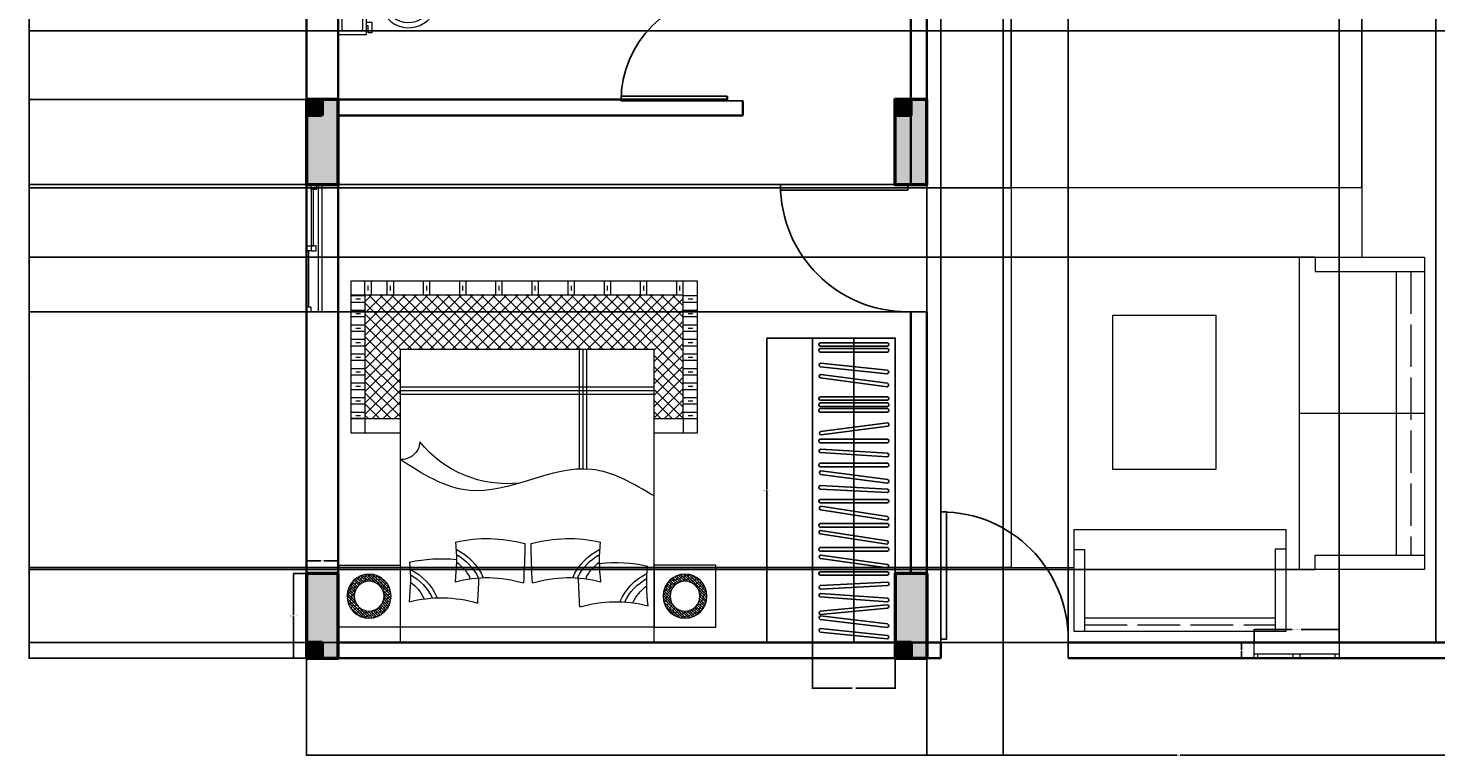
# Model space of a CAD drawing. Units: inches. Extents: x 393 to 993, y 153 to 660.
# Tile 1 of 6: x 393 to 791, y 153 to 359. Entities that reach past the tile are written whole.
import ezdxf

# ---------------------------------------------------------------- set-up
doc = ezdxf.new("R2010")
doc.units = ezdxf.units.IN
doc.header["$MEASUREMENT"] = 0
doc.linetypes.add('ACAD_ISO02W100', pattern=[15, 12, -3])
for name, color, linetype, lineweight in [('A-ANNO-DIMS', 2, 'Continuous', 18), ('A-COLS', 40, 'Continuous', 50), ('A-FLOR-CASE', 72, 'Continuous', 25), ('A-FLOR-FIXT', 9, 'Continuous', 18), ('A-FURN-HIDN', 72, 'ACAD_ISO02W100', 13), ('A-GLAZ', 4, 'Continuous', 20), ('A-WALL', 40, 'Continuous', 35), ('DOORS', 32, 'Continuous', 25), ('FURNITURE', 72, 'Continuous', 18)]:
    doc.layers.add(name, color=color, linetype=linetype, lineweight=lineweight)
doc.styles.get("Standard").update_dxf_attribs({"font": 'arial.ttf'})
doc.dimstyles.get("Standard").update_dxf_attribs({"dimtxt": 0.18, "dimasz": 0.18, "dimexe": 0.18, "dimexo": 0.0625, "dimgap": 0.09, "dimtad": 0, "dimtih": 1, "dimtoh": 1, "dimdec": 1, "dimzin": 0, "dimdsep": 46, "dimlunit": 3, "dimtxsty": 'Standard', "dimcen": 0.09, "dimadec": 0, "dimazin": 0, "dimtfac": 1, "dimtdec": 1, "dimtofl": 0, "dimtmove": 0, "dimatfit": 3, "dimfxl": 1, "dimtolj": 1, "dimtzin": 0, "dimarcsym": 0})

# ---------------------------------------------------------------- blocks, each defined once
blk = doc.blocks.new('W')
for p, q in [((518.15, 606.48), (554.15, 606.48)), ((518.15, 605.48), (554.15, 605.48))]:
    blk.add_line(p, q)
for points in [[(518.15, 609.91), (554.15, 609.91), (554.15, 600.91), (518.15, 600.91)], [(519.42, 609.91), (518.15, 609.91), (518.15, 608.51), (519.42, 608.51)], [(519.42, 609.91), (535.35, 609.91), (535.35, 609.3), (519.42, 609.3)], [(535.35, 609.91), (536.78, 609.91), (536.78, 608.51), (535.35, 608.51)], [(536.78, 608.51), (535.35, 608.51), (535.35, 607.12), (536.78, 607.12)], [(552.72, 608.51), (536.78, 608.51), (536.78, 607.91), (552.72, 607.91)], [(552.72, 608.51), (554.15, 608.51), (554.15, 607.12), (552.72, 607.12)]]:
    blk.add_lwpolyline(points, close=True)
blk = doc.blocks.new('*U3')
for p, q in [((0, 0), (0, -6)), ((40, 0), (40, -6))]:
    blk.add_line(p, q)
blk.add_lwpolyline([(0, 0), (0, 40), (1.75, 40), (1.75, 0)], close=True)
blk.add_arc((0, 0), 40, 0, 90)
blk = doc.blocks.new('GG')
for p, q in [((752.1, 182.21), (764.1, 182.21)), ((752.96, 182.21), (752.96, 180.91)), ((763, 180.91), (763, 182.21))]:
    blk.add_line(p, q)
for points in [[(740.1, 180.91), (740.1, 185.41), (764.1, 185.41), (764.1, 180.91), (740.1, 180.91), (740.1, 182.21), (752.1, 182.21)], [(740.1, 180.91), (741.16, 180.91), (741.16, 182.21)], [(752.1, 180.91), (751.16, 180.91), (751.16, 182.21)]]:
    blk.add_lwpolyline(points)
blk = doc.blocks.new('BED')
h = blk.add_hatch()
h.set_pattern_fill('ANSI38', color=256, scale=4.4)
h.paths.add_polyline_path([(503.33, 587.82, 1), (515.77, 587.82, 1)])
h.paths.add_polyline_path([(513.77, 587.82, -1), (505.33, 587.82, -1)], flags=16)
h = blk.add_hatch()
h.set_pattern_fill('ANSI38', color=256, scale=4.4)
h.paths.add_polyline_path([(592.69, 587.82, 1), (605.13, 587.82, 1)])
h.paths.add_polyline_path([(603.13, 587.82, -1), (594.69, 587.82, -1)], flags=16)
h = blk.add_hatch()
h.set_pattern_fill('ANSI37', color=256, scale=18)
h.paths.add_polyline_path([(518.29, 518.09), (518.29, 537.6), (508.38, 537.6), (508.38, 502.74), (598.4, 502.74), (598.4, 537.6), (590.17, 537.6), (590.17, 518.09)])
for p, q in [((569.1, 551.87), (569.1, 518.09)), ((570.1, 551.87), (570.1, 518.09)), ((571.1, 551.87), (571.1, 518.09)), ((508.38, 537.6), (508.38, 541.6)), ((598.4, 537.6), (598.4, 541.6)), ((508.38, 537.6), (504.38, 537.6)), ((504.38, 537.6), (508.38, 537.6)), ((598.4, 537.6), (602.4, 537.6)), ((504.38, 535.78), (508.38, 535.78)), ((505.75, 536.69), (507.09, 536.69)), ((598.4, 535.78), (602.4, 535.78)), ((599.77, 536.69), (601.11, 536.69)), ((504.38, 533.48), (508.38, 533.48)), ((504.38, 531.66), (508.38, 531.66)), ((505.75, 532.57), (507.09, 532.57)), ((518.29, 530.67), (590.17, 530.67)), ((518.29, 529.67), (590.17, 529.67)), ((598.4, 533.48), (602.4, 533.48)), ((598.4, 531.66), (602.4, 531.66)), ((599.77, 532.57), (601.11, 532.57)), ((504.38, 529.37), (508.38, 529.37)), ((504.38, 527.54), (508.38, 527.54)), ((505.75, 528.46), (507.09, 528.46)), ((518.29, 528.67), (590.17, 528.67)), ((598.4, 529.37), (602.4, 529.37)), ((598.4, 527.54), (602.4, 527.54)), ((599.77, 528.46), (601.11, 528.46)), ((504.38, 525.25), (508.38, 525.25)), ((504.38, 523.43), (508.38, 523.43)), ((505.75, 524.34), (507.09, 524.34)), ((598.4, 525.25), (602.4, 525.25)), ((598.4, 523.43), (602.4, 523.43)), ((599.77, 524.34), (601.11, 524.34)), ((504.38, 521.13), (508.38, 521.13)), ((504.38, 519.31), (508.38, 519.31)), ((505.75, 520.22), (507.09, 520.22)), ((598.4, 521.13), (602.4, 521.13)), ((598.4, 519.31), (602.4, 519.31)), ((599.77, 520.22), (601.11, 520.22)), ((504.38, 517.02), (508.38, 517.02)), ((504.38, 515.19), (508.38, 515.19)), ((505.75, 516.11), (507.09, 516.11)), ((598.4, 517.02), (602.4, 517.02)), ((598.4, 515.19), (602.4, 515.19)), ((599.77, 516.11), (601.11, 516.11)), ((504.38, 512.9), (508.38, 512.9)), ((504.38, 511.08), (508.38, 511.08)), ((505.75, 511.99), (507.09, 511.99)), ((598.4, 512.9), (602.4, 512.9)), ((598.4, 511.08), (602.4, 511.08)), ((599.77, 511.99), (601.11, 511.99)), ((504.38, 508.78), (508.38, 508.78)), ((504.38, 506.96), (508.38, 506.96)), ((505.75, 507.87), (507.09, 507.87)), ((598.4, 508.78), (602.4, 508.78)), ((598.4, 506.96), (602.4, 506.96)), ((599.77, 507.87), (601.11, 507.87)), ((504.38, 504.67), (508.38, 504.67)), ((504.38, 502.84), (508.38, 502.84)), ((508.38, 502.74), (504.38, 502.74)), ((505.75, 503.76), (507.09, 503.76)), ((508.38, 502.74), (508.38, 498.74)), ((510.2, 502.74), (510.2, 498.74)), ((514.7, 502.74), (514.7, 498.74)), ((516.52, 502.74), (516.52, 498.74)), ((524.93, 502.74), (524.93, 498.74)), ((526.76, 502.74), (526.76, 498.74)), ((535.17, 502.74), (535.17, 498.74)), ((536.99, 502.74), (536.99, 498.74)), ((545.4, 502.74), (545.4, 498.74)), ((547.22, 502.74), (547.22, 498.74)), ((555.64, 502.74), (555.64, 498.74)), ((557.46, 502.74), (557.46, 498.74)), ((565.87, 502.74), (565.87, 498.74)), ((567.69, 502.74), (567.69, 498.74)), ((576.11, 502.74), (576.11, 498.74)), ((577.93, 502.74), (577.93, 498.74)), ((586.34, 502.74), (586.34, 498.74)), ((588.16, 502.74), (588.16, 498.74)), ((596.58, 502.74), (596.58, 498.74)), ((598.4, 504.67), (602.4, 504.67)), ((598.4, 502.84), (602.4, 502.84)), ((598.4, 502.74), (598.4, 498.74)), ((599.77, 503.76), (601.11, 503.76)), ((509.29, 501.37), (509.29, 500.03)), ((515.61, 501.37), (515.61, 500.03)), ((525.84, 501.37), (525.84, 500.03)), ((536.08, 501.37), (536.08, 500.03)), ((546.31, 501.37), (546.31, 500.03)), ((556.55, 501.37), (556.55, 500.03)), ((566.78, 501.37), (566.78, 500.03)), ((577.02, 501.37), (577.02, 500.03)), ((587.25, 501.37), (587.25, 500.03)), ((597.49, 501.37), (597.49, 500.03))]:
    blk.add_line(p, q)
for points in [[(518.29, 600.91), (590.17, 600.91), (590.17, 518.09), (518.29, 518.09)], [(518.29, 600.91), (590.17, 600.91), (590.17, 596.58), (518.29, 596.58)], [(518.29, 596.58), (500.81, 596.58), (500.81, 579.05), (518.29, 579.05)], [(590.17, 596.58), (607.65, 596.58), (607.65, 579.05), (590.17, 579.05)]]:
    blk.add_lwpolyline(points, close=True)
for points in [[(590.17, 541.6), (602.4, 541.6), (602.4, 498.74), (504.38, 498.74), (504.38, 541.6), (518.29, 541.6)], [(590.17, 537.6), (598.4, 537.6), (598.4, 502.74), (508.38, 502.74), (508.38, 537.6), (518.29, 537.6)]]:
    blk.add_lwpolyline(points)
for centre, radius in [((509.55, 587.82), 6.22), ((598.91, 587.82), 6.22), ((509.55, 587.82), 4.22), ((598.91, 587.82), 4.22)]:
    blk.add_circle(centre, radius)
for centre, radius, start, end in [((529.91, 624.74), 36.45, 255.5916, 286.3549), ((470.26, 583.22), 50.97, 354.3497, 7.0055), ((355.3, 577.59), 185.28, 1.5729, 3.7686), ((754.03, 578.68), 185.28, 176.2314, 178.7587), ((579.42, 625.84), 36.45, 253.6451, 284.4084), ((595.11, 595.65), 15.87, 203.1669, 244.1569), ((595.11, 595.65), 14.59, 205.0537, 241.3945), ((595.75, 595.21), 12.82, 205.4838, 233.4213), ((639.07, 584.32), 50.97, 172.9945, 185.6503), ((514.22, 594.55), 15.87, 295.8431, 336.8331), ((514.22, 594.55), 14.59, 298.6055, 334.9463), ((513.58, 594.12), 12.82, 306.5787, 334.5162), ((542.93, 619.04), 36.45, 255.5916, 286.3549), ((483.27, 577.52), 50.97, 354.3497, 7.0055), ((527.24, 588.86), 15.87, 295.8431, 336.8331), ((527.24, 588.86), 14.59, 298.6055, 334.9463), ((526.6, 588.42), 12.82, 306.5787, 334.5162), ((368.32, 571.89), 185.28, 0.3263, 3.7686), ((740.67, 571.89), 185.28, 176.2314, 179.6737), ((566.06, 619.04), 36.45, 253.6451, 284.4084), ((581.75, 588.86), 15.87, 203.1669, 244.1569), ((581.75, 588.86), 14.59, 205.0537, 241.3945), ((582.39, 588.42), 12.82, 205.4838, 233.4213), ((625.71, 577.52), 50.97, 172.9945, 185.6503), ((529.89, 618.01), 40.79, 257.3847, 276.1312), ((579.44, 619.11), 40.79, 263.4008, 282.6153), ((542.91, 612.32), 40.79, 257.3847, 285.1893), ((566.08, 612.32), 40.79, 254.8107, 282.6153), ((548.65, 524.17), 31.85, 83.7477, 141.0207), ((518.63, 543.94), 5.27, 2.9325, 93.7021)]:
    blk.add_arc(centre, radius, start, end)
blk.add_open_spline([(590.17, 559.5), (584.37, 556.05), (568.03, 546.36), (541.55, 563.96), (524.71, 553.27), (518.29, 549.19)], degree=3, knots=[0, 0, 0, 0, 19.259502, 54.250447, 75.777559, 75.777559, 75.777559, 75.777559])
blk = doc.blocks.new('COOB')
blk.add_line((626.78, 600.91), (626.78, 514.86))
blk.add_lwpolyline([(638.48, 600.91), (615.08, 600.91), (615.08, 514.86), (638.48, 514.86)], close=True)
for points in [[(636.21, 599.92), (617.25, 598)], [(617.35, 597.01), (636.31, 598.93)], [(636.17, 596.68), (617.24, 594.42)], [(617.36, 593.43), (636.28, 595.69)], [(636.24, 589.41), (617.23, 588.06)], [(617.24, 592.05), (636.21, 590.25)], [(636.31, 591.25), (617.34, 593.04)], [(617.31, 587.07), (636.32, 588.41)], [(636.35, 584.83), (617.32, 585.82)], [(636.31, 581.92), (617.25, 581.92)], [(617.26, 584.82), (636.29, 583.84)], [(617.25, 580.92), (636.31, 580.92)], [(636.15, 579.82), (617.28, 577.19)], [(617.41, 576.2), (636.29, 578.83)], [(636.31, 575.1), (617.25, 575.1)], [(617.25, 574.1), (636.31, 574.1)], [(636.04, 573.13), (617.21, 570.23)], [(617.36, 569.24), (636.2, 572.14)], [(636.31, 568.28), (617.25, 568.28)], [(617.25, 567.28), (636.31, 567.28)], [(636.12, 566.32), (617.28, 563.41)], [(617.44, 562.42), (636.27, 565.34)], [(636.25, 558.53), (617.21, 557.57)], [(636.31, 561.46), (617.25, 561.46)], [(617.25, 560.46), (636.31, 560.46)], [(617.26, 556.57), (636.3, 557.54)], [(636.23, 555.87), (617.33, 553.42)], [(617.46, 552.43), (636.36, 554.88)], [(636.31, 551.24), (617.25, 551.24)], [(617.25, 550.24), (636.31, 550.24)], [(636.26, 548.43), (617.24, 547.23)], [(617.3, 546.23), (636.32, 547.43)], [(636.31, 544.42), (617.25, 544.42)], [(617.25, 543.42), (636.31, 543.42)], [(636.36, 539.77), (617.46, 542.23)], [(617.33, 541.23), (636.23, 538.78)], [(636.31, 535.8), (617.25, 535.8)], [(617.25, 534.8), (636.31, 534.8)], [(636.31, 534.19), (617.25, 534.19)], [(617.25, 533.19), (636.31, 533.19)], [(636.31, 532.44), (617.25, 532.44)], [(617.25, 531.44), (636.31, 531.44)], [(636.16, 528.62), (617.27, 526.12)], [(617.4, 525.13), (636.29, 527.62)], [(636.19, 524.96), (617.24, 522.96)], [(617.35, 521.97), (636.3, 523.96)], [(636.31, 518.8), (617.25, 518.8)], [(617.25, 517.8), (636.31, 517.8)], [(636.31, 517.14), (617.25, 517.14)], [(617.25, 516.14), (636.31, 516.14)]]:
    blk.add_lwpolyline(points)
for centre, start, end in [((617.44, 597.52), 111.987, 259.5876), ((636.11, 599.41), 291.987, 79.5876), ((617.45, 593.94), 113.0233, 260.6239), ((636.08, 596.17), 293.0233, 80.6239), ((617.43, 592.53), 100.7874, 248.388), ((636.12, 590.76), 280.7874, 68.388), ((636.13, 588.9), 290.2473, 77.8479), ((617.41, 587.58), 110.2473, 257.8479), ((617.43, 585.31), 103.2278, 250.8284), ((617.4, 581.42), 106.1997, 253.8003), ((636.18, 584.34), 283.2278, 70.8284), ((636.16, 581.42), 286.1997, 73.8003), ((636.08, 579.31), 294.1332, 81.7338), ((617.4, 574.6), 106.1997, 253.8003), ((617.49, 576.72), 114.1332, 261.7338), ((636.16, 574.6), 286.1997, 73.8003), ((617.43, 569.76), 114.9436, 262.5442), ((635.98, 572.61), 294.9436, 82.5442), ((617.4, 567.78), 106.1997, 253.8003), ((636.05, 565.81), 294.9996, 82.6002), ((636.16, 567.78), 286.1997, 73.8003), ((617.5, 562.94), 114.9996, 262.6002), ((617.38, 557.08), 109.0898, 256.6904), ((617.4, 560.96), 106.1997, 253.8003), ((636.13, 558.03), 289.0898, 76.6904), ((636.16, 560.96), 286.1997, 73.8003), ((636.15, 555.36), 293.5955, 81.1961), ((617.4, 550.74), 106.1997, 253.8003), ((617.54, 552.94), 113.5955, 261.1961), ((636.16, 550.74), 286.1997, 73.8003), ((617.41, 546.74), 109.8088, 257.4094), ((636.14, 547.92), 289.8088, 77.4094), ((617.4, 543.92), 106.1997, 253.8003), ((617.54, 541.71), 98.8065, 246.4071), ((636.16, 543.92), 286.1997, 73.8003), ((636.15, 539.3), 278.8065, 66.4071), ((617.4, 535.3), 106.1997, 253.8003), ((617.4, 533.69), 106.1997, 253.8003), ((636.16, 535.3), 286.1997, 73.8003), ((636.16, 533.69), 286.1997, 73.8003), ((617.4, 531.94), 106.1997, 253.8003), ((636.16, 531.94), 286.1997, 73.8003), ((617.48, 525.64), 113.7284, 261.329), ((636.08, 528.1), 293.7284, 81.329), ((617.44, 522.48), 112.2058, 259.8064), ((636.1, 524.44), 292.2058, 79.8064), ((617.4, 518.3), 106.1997, 253.8003), ((636.16, 518.3), 286.1997, 73.8003), ((617.4, 516.64), 106.1997, 253.8003), ((636.16, 516.64), 286.1997, 73.8003)]:
    blk.add_arc(centre, 0.521, start, end)
blk = doc.blocks.new('*U11')
for p, q in [((9.5, -6), (9.5, -2)), ((-10, -8.5), (-8, -8.5)), ((-10, -9.5), (-10, -8.5)), ((-7, -9.5), (-10, -9.5)), ((-8, -8.5), (-8, -8)), ((-7, -8), (-7, -9.5)), ((-4, -8), (-6, -14)), ((4, -8), (6, -14)), ((4, -14), (-4, -14))]:
    blk.add_line(p, q)
blk.add_lwpolyline([(10.5, -8), (10.5, 0), (-10.5, 0), (-10.5, -8)], close=True)
for points in [[(-9.5, -2), (-9.5, -6)], [(8.5, -1), (-8.5, -1)], [(-8.5, -7), (8.5, -7)]]:
    blk.add_lwpolyline(points)
for centre, radius, start, end in [((-8.625, -1.875), 0.8839, 81.8699, 188.1301), ((8.625, -1.875), 0.8839, 351.8699, 98.1301), ((-8.625, -6.125), 0.8839, 171.869898, 278.1301), ((8.625, -6.125), 0.8839, 261.8699, 8.1301), ((-0.4772, -19.9188), 8.0953, 133.01722, 273.38), ((0.0374, -19.8731), 7.127, 124.50543, 269.7), ((-0.0373, -19.8731), 7.127, 270.3, 55.4946), ((0.4773, -19.9188), 8.0953, 266.62, 46.9828)]:
    blk.add_arc(centre, radius, start, end)
blk = doc.blocks.new('COL-9X24-LH')
h = blk.add_hatch(color=256)
h.dxf.hatch_style = 1
h.paths.add_polyline_path([(4.5, 24), (0, 24), (0, 19.5), (4.5, 19.5)])
h = blk.add_hatch(color=256)
h.dxf.hatch_style = 1
h.paths.add_polyline_path([(4.5, 19.5), (0, 19.5), (0, 0), (9, 0), (9, 24), (4.5, 24)])
for p, q in [((4.5, 24), (0, 24)), ((0, 24), (0, 19.5)), ((4.5, 24), (4.5, 19.5)), ((4.5, 19.5), (0, 19.5))]:
    blk.add_line(p, q)
blk.add_lwpolyline([(9, 24), (0, 24), (0, 0), (9, 0), (9, 24)])
blk = doc.blocks.new('COL-9X24-END')
h = blk.add_hatch(color=256)
h.dxf.hatch_style = 1
h.paths.add_polyline_path([(9, 24), (0, 24), (0, 4.5), (4.5, 4.5), (4.5, 0), (9, 0)])
h = blk.add_hatch(color=256)
h.dxf.hatch_style = 1
h.paths.add_polyline_path([(4.5, 4.5), (0, 4.5), (0, 0), (4.5, 0)])
for p, q in [((4.5, 4.5), (0, 4.5)), ((0, 4.5), (0, 0)), ((0, 4.5), (4.5, 4.5)), ((4.5, 4.5), (4.5, 0)), ((4.5, 0), (0, 0))]:
    blk.add_line(p, q)
blk.add_lwpolyline([(9, 24), (0, 24), (0, 0), (9, 0), (9, 24)])
blk = doc.blocks.new('*D22')
at = {"layer": 'A-ANNO-DIMS', "color": 0, "lineweight": -2, "transparency": 16777216}
for p, q in [((471.92, 204.91), (468.2, 204.91)), ((468.38, 204.73), (468.38, 193.09)), ((468.38, 181.09), (468.38, 192.72)), ((471.92, 180.91), (468.2, 180.91))]:
    blk.add_line(p, q, dxfattribs=at)
at = {"layer": 'A-ANNO-DIMS', "color": 0, "transparency": 16777216}
for points in [[(468.35, 204.73), (468.41, 204.73), (468.38, 204.91)], [(468.35, 181.09), (468.41, 181.09), (468.38, 180.91)]]:
    blk.add_solid(points, dxfattribs=at)
at = {"layer": 'Defpoints', "color": 0, "transparency": 16777216}
for p in [(468.38, 204.91), (471.98, 204.91), (471.98, 180.91)]:
    blk.add_point(p, dxfattribs=at)
at = {"layer": 'A-ANNO-DIMS', "color": 0, "transparency": 16777216, "insert": (468.38, 192.91), "char_height": 0.18, "attachment_point": 5}
blk.add_mtext('\\A1;END COL. 24 TYP.', dxfattribs=at)
blk = doc.blocks.new('*D23')
at = {"layer": 'A-ANNO-DIMS', "color": 0, "lineweight": -2, "transparency": 16777216}
for p, q in [((471.98, 204.97), (471.98, 208.69)), ((472.16, 208.51), (476.02, 208.51)), ((480.8, 208.51), (476.94, 208.51)), ((480.98, 204.97), (480.98, 208.69))]:
    blk.add_line(p, q, dxfattribs=at)
at = {"layer": 'A-ANNO-DIMS', "color": 0, "transparency": 16777216}
for points in [[(472.16, 208.54), (472.16, 208.48), (471.98, 208.51)], [(480.8, 208.54), (480.8, 208.48), (480.98, 208.51)]]:
    blk.add_solid(points, dxfattribs=at)
at = {"layer": 'Defpoints', "color": 0, "transparency": 16777216}
for p in [(480.98, 208.51), (471.98, 204.91), (480.98, 204.91)]:
    blk.add_point(p, dxfattribs=at)
at = {"layer": 'A-ANNO-DIMS', "color": 0, "transparency": 16777216, "insert": (476.48, 208.51), "char_height": 0.18, "attachment_point": 5}
blk.add_mtext('\\A1;9 TYP.', dxfattribs=at)
blk = doc.blocks.new('*D30')
at = {"layer": 'A-ANNO-DIMS', "color": 0, "lineweight": -2, "transparency": 16777216}
for p, q in [((740.1, 185.47), (740.1, 189.19)), ((740.28, 189.01), (750.84, 189.01)), ((763.92, 189.01), (753.36, 189.01)), ((764.1, 185.47), (764.1, 189.19))]:
    blk.add_line(p, q, dxfattribs=at)
at = {"layer": 'A-ANNO-DIMS', "color": 0, "transparency": 16777216}
for points in [[(740.28, 189.04), (740.28, 188.98), (740.1, 189.01)], [(763.92, 189.04), (763.92, 188.98), (764.1, 189.01)]]:
    blk.add_solid(points, dxfattribs=at)
at = {"layer": 'Defpoints', "color": 0, "transparency": 16777216}
for p in [(764.1, 189.01), (740.1, 185.41), (764.1, 185.41)]:
    blk.add_point(p, dxfattribs=at)
at = {"layer": 'A-ANNO-DIMS', "color": 0, "transparency": 16777216, "insert": (752.1, 189.01), "char_height": 0.18, "attachment_point": 5}
blk.add_mtext('\\A1;ENTRY WINDOW 24', dxfattribs=at)
blk = doc.blocks.new('*D31')
at = {"layer": 'A-ANNO-DIMS', "color": 0, "lineweight": -2, "transparency": 16777216}
for p, q in [((740.04, 185.41), (736.32, 185.41)), ((736.5, 185.23), (736.5, 183.34)), ((740.04, 180.91), (736.32, 180.91)), ((736.5, 181.09), (736.5, 182.98))]:
    blk.add_line(p, q, dxfattribs=at)
at = {"layer": 'A-ANNO-DIMS', "color": 0, "transparency": 16777216}
for points in [[(736.47, 185.23), (736.53, 185.23), (736.5, 185.41)], [(736.47, 181.09), (736.53, 181.09), (736.5, 180.91)]]:
    blk.add_solid(points, dxfattribs=at)
at = {"layer": 'Defpoints', "color": 0, "transparency": 16777216}
for p in [(736.5, 185.41), (740.1, 185.41), (740.1, 180.91)]:
    blk.add_point(p, dxfattribs=at)
at = {"layer": 'A-ANNO-DIMS', "color": 0, "transparency": 16777216, "insert": (736.5, 183.16), "char_height": 0.18, "attachment_point": 5}
blk.add_mtext('\\A1;5', dxfattribs=at)
blk = doc.blocks.new('*D34')
at = {"layer": 'A-ANNO-DIMS', "color": 0, "lineweight": -2, "transparency": 16777216}
for p, q in [((615.11, 271.45), (602.09, 271.45)), ((602.27, 271.27), (602.27, 228.61)), ((602.27, 185.59), (602.27, 228.25)), ((615.11, 185.41), (602.09, 185.41))]:
    blk.add_line(p, q, dxfattribs=at)
at = {"layer": 'A-ANNO-DIMS', "color": 0, "transparency": 16777216}
for points in [[(602.24, 271.27), (602.3, 271.27), (602.27, 271.45)], [(602.24, 185.59), (602.3, 185.59), (602.27, 185.41)]]:
    blk.add_solid(points, dxfattribs=at)
at = {"layer": 'Defpoints', "color": 0, "transparency": 16777216}
for p in [(615.18, 271.45), (602.27, 185.41), (615.18, 185.41)]:
    blk.add_point(p, dxfattribs=at)
at = {"layer": 'A-ANNO-DIMS', "color": 0, "transparency": 16777216, "insert": (602.27, 228.43), "char_height": 0.18, "attachment_point": 5}
blk.add_mtext('\\A1;WARDROBE 86 TYP.', dxfattribs=at)
blk = doc.blocks.new('*D35')
at = {"layer": 'A-ANNO-DIMS', "color": 0, "lineweight": -2, "transparency": 16777216}
for p, q in [((615.18, 185.34), (615.18, 172.32)), ((638.58, 185.34), (638.58, 172.32)), ((615.36, 172.5), (626.35, 172.5)), ((638.4, 172.5), (627.41, 172.5))]:
    blk.add_line(p, q, dxfattribs=at)
at = {"layer": 'A-ANNO-DIMS', "color": 0, "transparency": 16777216}
for points in [[(615.36, 172.53), (615.36, 172.47), (615.18, 172.5)], [(638.4, 172.53), (638.4, 172.47), (638.58, 172.5)]]:
    blk.add_solid(points, dxfattribs=at)
at = {"layer": 'Defpoints', "color": 0, "transparency": 16777216}
for p in [(615.18, 185.41), (638.58, 185.41), (638.58, 172.5)]:
    blk.add_point(p, dxfattribs=at)
at = {"layer": 'A-ANNO-DIMS', "color": 0, "transparency": 16777216, "insert": (626.88, 172.5), "char_height": 0.18, "attachment_point": 5}
blk.add_mtext('\\A1;23 TYP.', dxfattribs=at)
blk = doc.blocks.new('*D44')
at = {"layer": 'A-ANNO-DIMS', "color": 0, "lineweight": -2, "transparency": 16777216}
for p, q in [((471.98, 180.84), (471.98, 153.33)), ((965.48, 180.84), (965.48, 153.33)), ((472.16, 153.51), (718.33, 153.51)), ((965.3, 153.51), (719.13, 153.51))]:
    blk.add_line(p, q, dxfattribs=at)
at = {"layer": 'A-ANNO-DIMS', "color": 0, "transparency": 16777216}
for points in [[(472.16, 153.54), (472.16, 153.48), (471.98, 153.51)], [(965.3, 153.54), (965.3, 153.48), (965.48, 153.51)]]:
    blk.add_solid(points, dxfattribs=at)
at = {"layer": 'Defpoints', "color": 0, "transparency": 16777216}
for p in [(471.98, 180.91), (965.48, 180.91), (965.48, 153.51)]:
    blk.add_point(p, dxfattribs=at)
at = {"layer": 'A-ANNO-DIMS', "color": 0, "transparency": 16777216, "insert": (718.73, 153.51), "char_height": 0.18, "attachment_point": 5}
blk.add_mtext('\\A1;493.5', dxfattribs=at)
blk = doc.blocks.new('*D51')
at = {"layer": 'A-ANNO-DIMS', "color": 0, "lineweight": -2, "transparency": 16777216}
for p, q in [((471.92, 338.91), (393.4, 338.91)), ((393.58, 338.73), (393.58, 260.09)), ((393.58, 181.09), (393.58, 259.72)), ((471.92, 180.91), (393.4, 180.91))]:
    blk.add_line(p, q, dxfattribs=at)
at = {"layer": 'A-ANNO-DIMS', "color": 0, "transparency": 16777216}
for points in [[(393.55, 338.73), (393.61, 338.73), (393.58, 338.91)], [(393.55, 181.09), (393.61, 181.09), (393.58, 180.91)]]:
    blk.add_solid(points, dxfattribs=at)
at = {"layer": 'Defpoints', "color": 0, "transparency": 16777216}
for p in [(393.58, 338.91), (471.98, 338.91), (471.98, 180.91)]:
    blk.add_point(p, dxfattribs=at)
at = {"layer": 'A-ANNO-DIMS', "color": 0, "transparency": 16777216, "insert": (393.58, 259.91), "char_height": 0.18, "attachment_point": 5}
blk.add_mtext('\\A1;158', dxfattribs=at)
blk = doc.blocks.new('*D52')
at = {"layer": 'A-ANNO-DIMS', "color": 0, "lineweight": -2, "transparency": 16777216}
for p, q in [((480.92, 397.41), (393.4, 397.41)), ((393.58, 397.23), (393.58, 368.34)), ((393.58, 339.09), (393.58, 367.97)), ((471.92, 338.91), (393.4, 338.91))]:
    blk.add_line(p, q, dxfattribs=at)
at = {"layer": 'A-ANNO-DIMS', "color": 0, "transparency": 16777216}
for points in [[(393.55, 397.23), (393.61, 397.23), (393.58, 397.41)], [(393.55, 339.09), (393.61, 339.09), (393.58, 338.91)]]:
    blk.add_solid(points, dxfattribs=at)
at = {"layer": 'Defpoints', "color": 0, "transparency": 16777216}
for p in [(393.58, 397.41), (480.98, 397.41), (471.98, 338.91)]:
    blk.add_point(p, dxfattribs=at)
at = {"layer": 'A-ANNO-DIMS', "color": 0, "transparency": 16777216, "insert": (393.58, 368.16), "char_height": 0.18, "attachment_point": 5}
blk.add_mtext('\\A1;58.5', dxfattribs=at)
blk = doc.blocks.new('*D59')
at = {"layer": 'A-ANNO-DIMS', "color": 0, "lineweight": -2, "transparency": 16777216}
for p, q in [((651.48, 185.47), (651.48, 660.49)), ((651.66, 660.31), (669.26, 660.31)), ((687.3, 660.31), (669.7, 660.31)), ((687.48, 185.47), (687.48, 660.49))]:
    blk.add_line(p, q, dxfattribs=at)
at = {"layer": 'A-ANNO-DIMS', "color": 0, "transparency": 16777216}
for points in [[(651.66, 660.34), (651.66, 660.28), (651.48, 660.31)], [(687.3, 660.34), (687.3, 660.28), (687.48, 660.31)]]:
    blk.add_solid(points, dxfattribs=at)
at = {"layer": 'Defpoints', "color": 0, "transparency": 16777216}
for p in [(687.48, 660.31), (651.48, 185.41), (687.48, 185.41)]:
    blk.add_point(p, dxfattribs=at)
at = {"layer": 'A-ANNO-DIMS', "color": 0, "transparency": 16777216, "insert": (669.48, 660.31), "char_height": 0.18, "attachment_point": 5}
blk.add_mtext('\\A1;36', dxfattribs=at)
blk = doc.blocks.new('*D60')
at = {"layer": 'A-ANNO-DIMS', "color": 0, "lineweight": -2, "transparency": 16777216}
for p, q in [((642.92, 314.91), (393.4, 314.91)), ((393.58, 314.73), (393.58, 297.09)), ((393.58, 279.09), (393.58, 296.72)), ((642.92, 278.91), (393.4, 278.91))]:
    blk.add_line(p, q, dxfattribs=at)
at = {"layer": 'A-ANNO-DIMS', "color": 0, "transparency": 16777216}
for points in [[(393.55, 314.73), (393.61, 314.73), (393.58, 314.91)], [(393.55, 279.09), (393.61, 279.09), (393.58, 278.91)]]:
    blk.add_solid(points, dxfattribs=at)
at = {"layer": 'Defpoints', "color": 0, "transparency": 16777216}
for p in [(393.58, 314.91), (642.98, 314.91), (642.98, 278.91)]:
    blk.add_point(p, dxfattribs=at)
at = {"layer": 'A-ANNO-DIMS', "color": 0, "transparency": 16777216, "insert": (393.58, 296.91), "char_height": 0.18, "attachment_point": 5}
blk.add_mtext('\\A1;36', dxfattribs=at)
blk = doc.blocks.new('*D68')
at = {"layer": 'A-ANNO-DIMS', "color": 0, "lineweight": -2, "transparency": 16777216}
for p, q in [((671.33, 314.02), (671.33, 660.49)), ((671.51, 660.31), (720.57, 660.31)), ((770.41, 660.31), (721.36, 660.31)), ((770.59, 314.02), (770.59, 660.49))]:
    blk.add_line(p, q, dxfattribs=at)
at = {"layer": 'A-ANNO-DIMS', "color": 0, "transparency": 16777216}
for points in [[(671.51, 660.34), (671.51, 660.28), (671.33, 660.31)], [(770.41, 660.34), (770.41, 660.28), (770.59, 660.31)]]:
    blk.add_solid(points, dxfattribs=at)
at = {"layer": 'Defpoints', "color": 0, "transparency": 16777216}
for p in [(770.59, 660.31), (671.33, 313.96), (770.59, 313.96)]:
    blk.add_point(p, dxfattribs=at)
at = {"layer": 'A-ANNO-DIMS', "color": 0, "transparency": 16777216, "insert": (720.96, 660.31), "char_height": 0.18, "attachment_point": 5}
blk.add_mtext('\\A1;99.26', dxfattribs=at)
blk = doc.blocks.new('*D69')
at = {"layer": 'A-ANNO-DIMS', "color": 0, "lineweight": -2, "transparency": 16777216}
for p, q in [((671.27, 313.96), (393.4, 313.96)), ((393.58, 313.78), (393.58, 260.44)), ((393.58, 206.73), (393.58, 260.07)), ((671.27, 206.55), (393.4, 206.55))]:
    blk.add_line(p, q, dxfattribs=at)
at = {"layer": 'A-ANNO-DIMS', "color": 0, "transparency": 16777216}
for points in [[(393.55, 313.78), (393.61, 313.78), (393.58, 313.96)], [(393.55, 206.73), (393.61, 206.73), (393.58, 206.55)]]:
    blk.add_solid(points, dxfattribs=at)
at = {"layer": 'Defpoints', "color": 0, "transparency": 16777216}
for p in [(393.58, 313.96), (671.33, 313.96), (671.33, 206.55)]:
    blk.add_point(p, dxfattribs=at)
at = {"layer": 'A-ANNO-DIMS', "color": 0, "transparency": 16777216, "insert": (393.58, 260.26), "char_height": 0.18, "attachment_point": 5}
blk.add_mtext('\\A1;107.4', dxfattribs=at)
blk = doc.blocks.new('*D71')
at = {"layer": 'A-ANNO-DIMS', "color": 0, "lineweight": -2, "transparency": 16777216}
for p, q in [((956.42, 358.41), (393.4, 358.41)), ((393.58, 358.23), (393.58, 272.09)), ((393.58, 185.59), (393.58, 271.72)), ((956.42, 185.41), (393.4, 185.41))]:
    blk.add_line(p, q, dxfattribs=at)
at = {"layer": 'A-ANNO-DIMS', "color": 0, "transparency": 16777216}
for points in [[(393.55, 358.23), (393.61, 358.23), (393.58, 358.41)], [(393.55, 185.59), (393.61, 185.59), (393.58, 185.41)]]:
    blk.add_solid(points, dxfattribs=at)
at = {"layer": 'Defpoints', "color": 0, "transparency": 16777216}
for p in [(393.58, 358.41), (956.48, 358.41), (956.48, 185.41)]:
    blk.add_point(p, dxfattribs=at)
at = {"layer": 'A-ANNO-DIMS', "color": 0, "transparency": 16777216, "insert": (393.58, 271.91), "char_height": 0.18, "attachment_point": 5}
blk.add_mtext('\\A1;173', dxfattribs=at)
blk = doc.blocks.new('*D75')
at = {"layer": 'A-ANNO-DIMS', "color": 0, "lineweight": -2, "transparency": 16777216}
for p, q in [((764.1, 185.47), (764.1, 660.49)), ((764.28, 660.31), (777.39, 660.31)), ((791.3, 660.31), (778.19, 660.31)), ((791.48, 185.47), (791.48, 660.49))]:
    blk.add_line(p, q, dxfattribs=at)
at = {"layer": 'A-ANNO-DIMS', "color": 0, "transparency": 16777216}
for points in [[(764.28, 660.34), (764.28, 660.28), (764.1, 660.31)], [(791.3, 660.34), (791.3, 660.28), (791.48, 660.31)]]:
    blk.add_solid(points, dxfattribs=at)
at = {"layer": 'Defpoints', "color": 0, "transparency": 16777216}
for p in [(791.48, 660.31), (764.1, 185.41), (791.48, 185.41)]:
    blk.add_point(p, dxfattribs=at)
at = {"layer": 'A-ANNO-DIMS', "color": 0, "transparency": 16777216, "insert": (777.79, 660.31), "char_height": 0.18, "attachment_point": 5}
blk.add_mtext('\\A1;27.38', dxfattribs=at)
blk = doc.blocks.new('*D81')
at = {"layer": 'A-ANNO-DIMS', "color": 0, "lineweight": -2, "transparency": 16777216}
for p, q in [((647.48, 397.34), (647.48, 153.33)), ((669.09, 397.94), (669.09, 153.33)), ((647.66, 153.51), (657.91, 153.51)), ((668.91, 153.51), (658.66, 153.51))]:
    blk.add_line(p, q, dxfattribs=at)
at = {"layer": 'A-ANNO-DIMS', "color": 0, "transparency": 16777216}
for points in [[(647.66, 153.54), (647.66, 153.48), (647.48, 153.51)], [(668.91, 153.54), (668.91, 153.48), (669.09, 153.51)]]:
    blk.add_solid(points, dxfattribs=at)
at = {"layer": 'Defpoints', "color": 0, "transparency": 16777216}
for p in [(647.48, 397.41), (669.09, 398.01), (669.09, 153.51)]:
    blk.add_point(p, dxfattribs=at)
at = {"layer": 'A-ANNO-DIMS', "color": 0, "transparency": 16777216, "insert": (658.29, 153.51), "char_height": 0.18, "attachment_point": 5}
blk.add_mtext('\\A1;21.61', dxfattribs=at)
blk = doc.blocks.new('*D83')
at = {"layer": 'A-ANNO-DIMS', "color": 0, "lineweight": -2, "transparency": 16777216}
for p, q in [((757.33, 294.34), (393.4, 294.34)), ((393.58, 294.16), (393.58, 250.38)), ((393.58, 206.25), (393.58, 250.02)), ((757.33, 206.07), (393.4, 206.07))]:
    blk.add_line(p, q, dxfattribs=at)
at = {"layer": 'A-ANNO-DIMS', "color": 0, "transparency": 16777216}
for points in [[(393.55, 294.16), (393.61, 294.16), (393.58, 294.34)], [(393.55, 206.25), (393.61, 206.25), (393.58, 206.07)]]:
    blk.add_solid(points, dxfattribs=at)
at = {"layer": 'Defpoints', "color": 0, "transparency": 16777216}
for p in [(393.58, 294.34), (757.39, 294.34), (757.39, 206.07)]:
    blk.add_point(p, dxfattribs=at)
at = {"layer": 'A-ANNO-DIMS', "color": 0, "transparency": 16777216, "insert": (393.58, 250.2), "char_height": 0.18, "attachment_point": 5}
blk.add_mtext('\\A1;88.27', dxfattribs=at)

msp = doc.modelspace()

# ---------------------------------------------------------------- linework, layer by layer
at = {"layer": 'A-FURN-HIDN'}
for p, q in [((784.4314, 290.3394), (784.4314, 210.0654)), ((692.1215, 190.36), (746.0569, 190.36))]:
    msp.add_line(p, q, dxfattribs=at)
at = {"layer": 'A-WALL'}
for p, q in [((471.9798, 609.9066), (471.9798, 180.9066)), ((647.4798, 397.4066), (647.4798, 314.9066)), ((480.9798, 392.9066), (480.9798, 180.9066)), ((642.9798, 392.9066), (642.9798, 314.9066)), ((480.9798, 338.9066), (590.9798, 338.9066)), ((590.9798, 339.8638), (590.9798, 338.9066)), ((595.4798, 338.5513), (595.4798, 334.4066)), ((480.9798, 334.4066), (595.4798, 334.4066)), ((642.9798, 278.9066), (642.9798, 204.9066)), ((647.4798, 278.9066), (647.4798, 180.9066)), ((480.9798, 185.4066), (651.4798, 185.4066)), ((647.4798, 185.4066), (651.4798, 185.4066)), ((651.4798, 185.4066), (651.4798, 180.9066)), ((687.4798, 185.4066), (956.4798, 185.4066)), ((471.9798, 180.9066), (651.4798, 180.9066)), ((687.4798, 180.9066), (965.4798, 180.9066))]:
    msp.add_line(p, q, dxfattribs=at)
at = {"layer": 'FURNITURE'}
for p, q in [((770.5908, 313.958), (671.3346, 313.958)), ((671.3346, 313.958), (671.3346, 206.5548)), ((770.5908, 294.3394), (770.5908, 313.958)), ((757.3877, 294.3394), (757.3877, 290.3394)), ((757.3877, 290.3394), (788.2934, 290.3394)), ((780.2446, 290.3394), (780.2446, 210.0654)), ((752.8882, 250.2024), (788.2934, 250.2024)), ((689.1215, 211.684), (692.1215, 211.684)), ((692.1215, 211.684), (692.1215, 188.4757)), ((749.0569, 211.7613), (746.0569, 211.7613)), ((746.0569, 211.7613), (746.0569, 188.4757)), ((757.3877, 206.0654), (757.3877, 210.0654)), ((757.3877, 210.0654), (788.2934, 210.0654)), ((671.3346, 206.5548), (689.1215, 206.5548)), ((746.0569, 192.2915), (692.1215, 192.2915))]:
    msp.add_line(p, q, dxfattribs=at)
for points in [[(752.8882, 294.3394), (788.2934, 294.3394), (788.2934, 206.0654), (752.8882, 206.0654)], [(700.0884, 277.9839), (729.2739, 277.9839), (729.2739, 234.3342), (700.0884, 234.3342)], [(689.1215, 217.3432), (749.0569, 217.3432), (749.0569, 188.4757), (689.1215, 188.4757)]]:
    msp.add_lwpolyline(points, close=True, dxfattribs=at)

# ---------------------------------------------------------------- block references
at = {"layer": 'A-COLS'}
for name, p in [('COL-9X24-LH', (471.98, 314.907)), ('COL-9X24-LH', (638.48, 314.907)), ('COL-9X24-END', (471.98, 180.907)), ('COL-9X24-END', (638.577, 180.907))]:
    msp.add_blockref(name, p, dxfattribs=at)
at = {"layer": 'A-FLOR-CASE', "xscale": -1, "rotation": 180}
msp.add_blockref('COOB', (0.097, 786.3133), dxfattribs=at)
at = {"layer": 'A-FLOR-FIXT', "rotation": 90}
msp.add_blockref('*U11', (480.9798, 367.8225), dxfattribs=at)
at = {"layer": 'A-GLAZ', "rotation": 90}
msp.add_blockref('W', (1081.8865, -239.2421), dxfattribs=at)
at = {"layer": 'A-GLAZ'}
msp.add_blockref('GG', (0, 0), dxfattribs=at)
at = {"layer": 'DOORS'}
for p, xscale, yscale, zscale, rotation in [((590.9798, 338.5513), 0.75, 0.75, 0.75, 90.00000000000031), ((642.0798, 314.9066), -0.9, 0.9, 0.9, 89.99999999999969)]:
    msp.add_blockref('*U3', p, dxfattribs=dict(at, xscale=xscale, yscale=yscale, zscale=zscale, rotation=rotation))
at = {"layer": 'DOORS', "xscale": 0.9, "yscale": 0.9, "zscale": 0.9}
msp.add_blockref('*U3', (651.4798, 186.3066), dxfattribs=at)
at = {"layer": 'FURNITURE', "xscale": -1, "rotation": 180}
msp.add_blockref('BED', (-19.8291, 786.3133), dxfattribs=at)

# ---------------------------------------------------------------- dimensions: what is measured, and where the dimension line sits
at = {"layer": 'A-ANNO-DIMS'}
for base, p1, p2, override, picture, middle in [((687.4798, 660.3066), (651.4798, 185.4066), (687.4798, 185.4066), {"dimdec": 0, "dimlfac": 1, "dimrnd": 0, "dimzin": 0, "dimdsep": 46, "dimlunit": 2}, '*D59', (669.4798, 660.3066)), ((770.5908, 660.3066), (671.3346, 313.958), (770.5908, 313.958), {"dimdec": 2, "dimlfac": 1, "dimrnd": 0, "dimzin": 0, "dimdsep": 46, "dimlunit": 2}, '*D68', (720.9627, 660.3066)), ((791.4798, 660.3066), (764.1009, 185.4066), (791.4798, 185.4066), {"dimdec": 2, "dimlfac": 1, "dimrnd": 0, "dimzin": 0, "dimdsep": 46, "dimlunit": 2}, '*D75', (777.7904, 660.3066)), ((669.0909, 153.5066), (647.4798, 397.4066), (669.0909, 398.0071), {"dimdec": 2, "dimlfac": 1, "dimrnd": 0, "dimzin": 0, "dimdsep": 46, "dimlunit": 2}, '*D81', (658.2853, 153.5066)), ((965.4798, 153.5066), (471.9798, 180.9066), (965.4798, 180.9066), {"dimdec": 1, "dimlfac": 1, "dimrnd": 0, "dimzin": 0, "dimdsep": 46, "dimlunit": 2}, '*D44', (718.7298, 153.5066))]:
    dim = msp.add_linear_dim(base=base, p1=p1, p2=p2, dimstyle='Standard', override=override, dxfattribs=at)
    dim.commit()
    dim.dimension.update_dxf_attribs({"geometry": picture, "text_midpoint": middle})
for base, p1, p2, override, picture, middle in [((393.5798, 397.4066), (471.9798, 338.9066), (480.9798, 397.4066), {"dimdec": 1, "dimlfac": 1, "dimrnd": 0, "dimzin": 0, "dimdsep": 46, "dimlunit": 2}, '*D52', (393.5798, 368.1566)), ((393.5798, 358.4066), (956.4798, 185.4066), (956.4798, 358.4066), {"dimdec": 0, "dimlfac": 1, "dimrnd": 0, "dimzin": 0, "dimdsep": 46, "dimlunit": 2}, '*D71', (393.5798, 271.9066)), ((393.5798, 338.9066), (471.9798, 180.9066), (471.9798, 338.9066), {"dimdec": 0, "dimlfac": 1, "dimrnd": 0, "dimzin": 0, "dimdsep": 46, "dimlunit": 2}, '*D51', (393.5798, 259.9066)), ((393.5798, 314.9066), (642.9798, 278.9066), (642.9798, 314.9066), {"dimdec": 0, "dimlfac": 1, "dimrnd": 0, "dimzin": 0, "dimdsep": 46, "dimlunit": 2}, '*D60', (393.5798, 296.9066)), ((393.5798, 313.958), (671.3346, 206.5548), (671.3346, 313.958), {"dimdec": 1, "dimlfac": 1, "dimrnd": 0, "dimzin": 0, "dimdsep": 46, "dimlunit": 2}, '*D69', (393.5798, 260.2564)), ((393.5798, 294.3394), (757.3877, 206.0654), (757.3877, 294.3394), {"dimdec": 2, "dimlfac": 1, "dimrnd": 0, "dimzin": 0, "dimdsep": 46, "dimlunit": 2}, '*D83', (393.5798, 250.2024)), ((736.5009002742, 185.406640311), (740.1009002742, 180.906640311), (740.1009002742, 185.406640311), {"dimdec": 0, "dimlfac": 1, "dimrnd": 0, "dimzin": 0, "dimdsep": 46, "dimlunit": 2}, '*D31', (736.5009002742, 183.156640311))]:
    dim = msp.add_linear_dim(base=base, p1=p1, p2=p2, angle=90, dimstyle='Standard', override=override, dxfattribs=at)
    dim.commit()
    dim.dimension.update_dxf_attribs({"geometry": picture, "text_midpoint": middle})
for base, p1, p2, angle, text, picture, middle in [((602.2682, 185.4066), (615.1753, 271.4539), (615.1753, 185.4066), 270, 'WARDROBE <> TYP.', '*D34', (602.2682, 228.4303)), ((468.3798, 204.9066), (471.9798, 180.9066), (471.9798, 204.9066), 90, 'END COL. <> TYP.', '*D22', (468.3798, 192.9066))]:
    dim = msp.add_linear_dim(base=base, p1=p1, p2=p2, angle=angle, text=text, dimstyle='Standard', override={"dimdec": 0, "dimlfac": 1, "dimrnd": 0, "dimzin": 0, "dimdsep": 46, "dimlunit": 2}, dxfattribs=at)
    dim.commit()
    dim.dimension.update_dxf_attribs({"geometry": picture, "text_midpoint": middle})
for base, p1, p2, text, picture, middle in [((480.9798, 208.5066), (471.9798, 204.9066), (480.9798, 204.9066), '<> TYP.', '*D23', (476.4798, 208.5066)), ((764.1009, 189.0066), (740.1009, 185.4066), (764.1009, 185.4066), 'ENTRY WINDOW <>', '*D30', (752.1009, 189.0066)), ((638.5768, 172.4995), (615.1753, 185.4066), (638.5768, 185.4066), '<> TYP.', '*D35', (626.8761, 172.4995))]:
    dim = msp.add_linear_dim(base=base, p1=p1, p2=p2, text=text, dimstyle='Standard', override={"dimdec": 0, "dimlfac": 1, "dimrnd": 0, "dimzin": 0, "dimdsep": 46, "dimlunit": 2}, dxfattribs=at)
    dim.commit()
    dim.dimension.update_dxf_attribs({"geometry": picture, "text_midpoint": middle})

doc.saveas('drawing.dxf')
